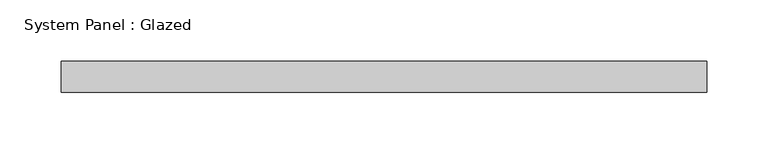
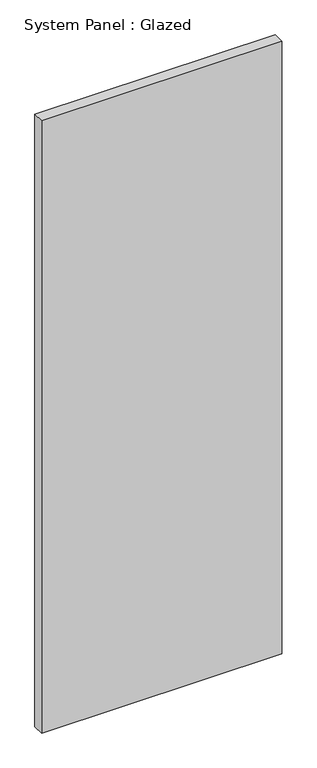
"""IFC4 building model written with IfcOpenShell, lengths in millimetres: plate geometry, System Panel : Glazed."""

from ifc_helpers import new_model, si_unit, origin, origin_with_axes, place, context, project, spatial, polyline, outline, extrude, source, transform, mapped, element, save


def system_panel_glazed_163e0323(model_context):
    return source(origin(), model_context, "Body", "SweptSolid", [
        extrude(outline(polyline([(262.5, 24.5), (-262.5, 24.5), (-262.5, 49.5), (262.5, 49.5), (262.5, 24.5)])), origin_with_axes(), (0.0, 0.0, 1.0), 1415.0),
    ])


if __name__ == "__main__":
    model = new_model("IFC4")
    model_context = context("Model", 3, world=origin())
    ifc_project = project(units=[si_unit("LENGTHUNIT", "METRE", prefix="MILLI")], contexts=[model_context])
    site = spatial("IfcSite", under=ifc_project)
    building = spatial("IfcBuilding", under=site)
    placement = place(None, origin())
    system_panel_glazed_shape = system_panel_glazed_163e0323(model_context)
    element("IfcPlate", 1, ObjectType="System Panel : Glazed", at=placement, inside=building, context=model_context, shape_type="MappedRepresentation", body=[
        mapped(system_panel_glazed_shape, transform((0.0, 0.0, 0.0), x_axis=(1.0, 0.0, 0.0), y_axis=(0.0, 1.0, 0.0), z_axis=(0.0, 0.0, 1.0))),
    ])
    save(model, "model.ifc")

# Revit data of these elements
# Type "System Panel : Glazed"
#   Construction Type Id = "GSP4R"
#   Analytic Construction = "1/8 in Pilkington single glazing"
#   Visual Light Transmittance = 0.9
#   Solar Heat Gain Coefficient = 0.86
#   Heat Transfer Coefficient (U) = 6.7069 W/(m²·K)
#   Define Thermal Properties by = 1
# Element 1 (IfcPlate, "System Panel : Glazed")
#   Materials on its faces: "Glass"
# Materials
#   "Glass": class "Glass", colour RGB 0 128 192, transparency 0.9, Description = "Soda Lime Glass", Cost = 0
